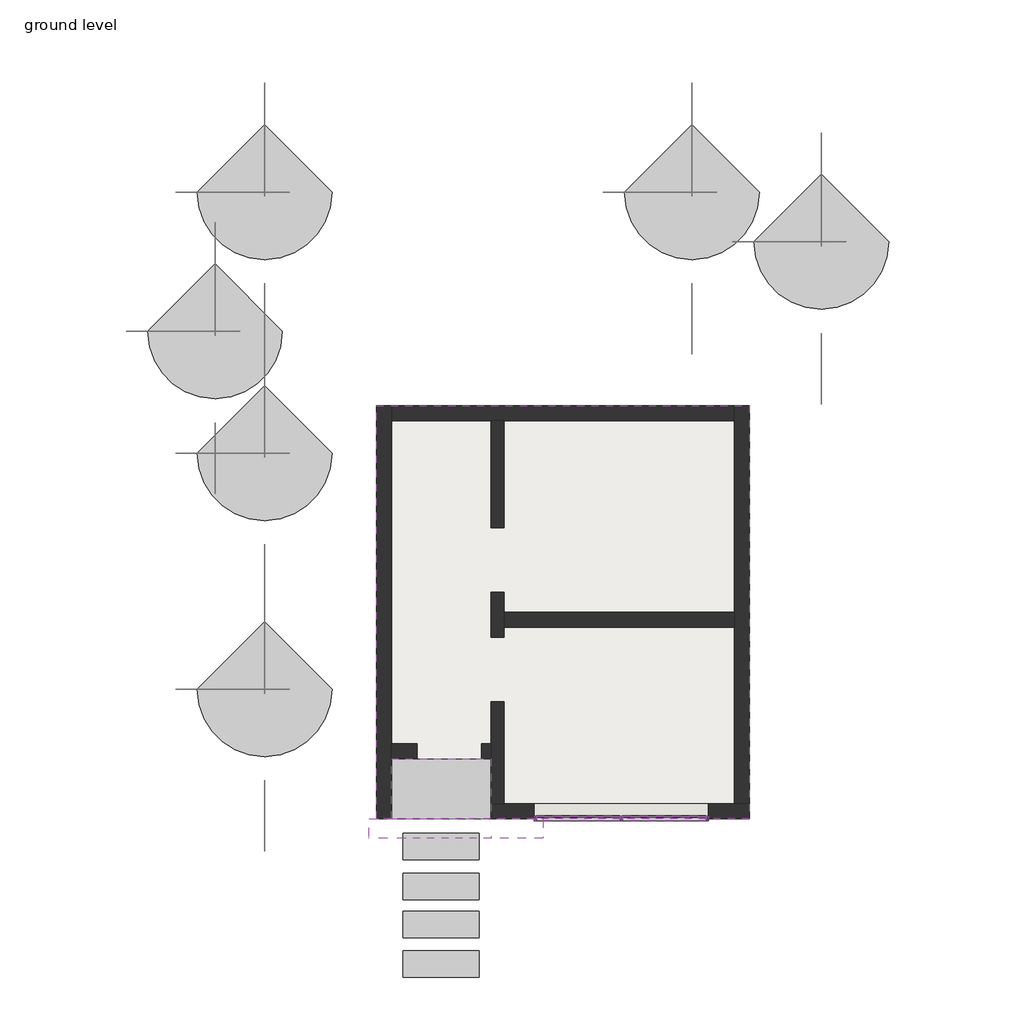
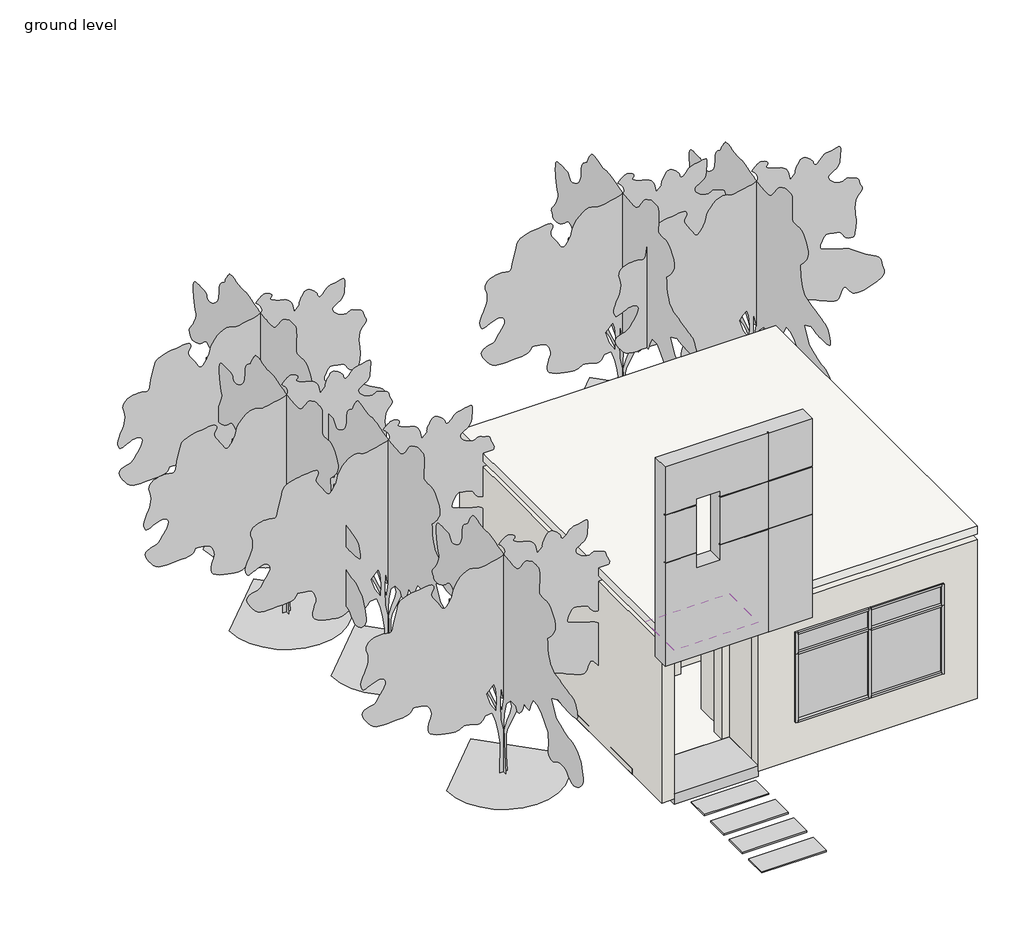
# One storey, incomplete: 12 members, 7 walls, 6 geographic elements, 4 plates, 3 proxies, 2 slabs, 1 covering.
"""IFC4 building model written with IfcOpenShell, lengths in millimetres."""

from ifc_helpers import new_model, si_unit, frame, origin, origin_with_axes, place, context, project, spatial, polyline, outline, extrude, faceted_brep, transform, mapped, element, save
from components import generic_models_2_generic_models_2_020848e7, generic_models_5_generic_models_5_6b2521d7, generic_models_6_generic_models_6_e57160bd, rpc_tree_deciduous_blue_berry_elder_15_a2d70376, member_9069d910, member_f8a7f713, member_03258ea9, member_54524429, member_711dd202, member_030f819f, system_panel_glazed_4e3b5d9d, system_panel_glazed_6984195a

model = new_model("IFC4")

# Units and contexts
model_context = context("Model", 3, world=origin())
ifc_project = project(units=[si_unit("LENGTHUNIT", "METRE", prefix="MILLI")], contexts=[model_context])

# Site, building, storey
site = spatial("IfcSite", under=ifc_project)
building = spatial("IfcBuilding", under=site)
storey = spatial("IfcBuildingStorey", under=building, Name="ground level", Elevation=0.0)

# Proxies
placement = place(None, origin())
generic_models_2_generic_models_2_shape = generic_models_2_generic_models_2_020848e7(model_context)
element("IfcBuildingElementProxy", 1, Name="Generic Models 2 : Generic Models 2", ObjectType="Generic Models 2 : Generic Models 2", at=placement, inside=storey, context=model_context, shape_type="MappedRepresentation", body=[
    mapped(generic_models_2_generic_models_2_shape, transform((0.0, 0.0, 0.0), x_axis=(1.0, 0.0, 0.0), y_axis=(0.0, 1.0, 0.0), z_axis=(0.0, 0.0, 1.0))),
])
generic_models_5_generic_models_5_shape = generic_models_5_generic_models_5_6b2521d7(model_context)
element("IfcBuildingElementProxy", 2, Name="Generic Models 5 : Generic Models 5", ObjectType="Generic Models 5 : Generic Models 5", at=placement, inside=storey, context=model_context, shape_type="MappedRepresentation", body=[
    mapped(generic_models_5_generic_models_5_shape, transform((0.0, 0.0, 0.0), x_axis=(1.0, 0.0, 0.0), y_axis=(0.0, 1.0, 0.0), z_axis=(0.0, 0.0, 1.0))),
])
generic_models_6_generic_models_6_shape = generic_models_6_generic_models_6_e57160bd(model_context)
element("IfcBuildingElementProxy", 3, Name="Generic Models 6 : Generic Models 6", ObjectType="Generic Models 6 : Generic Models 6", at=placement, inside=storey, context=model_context, shape_type="MappedRepresentation", body=[
    mapped(generic_models_6_generic_models_6_shape, transform((0.0, 0.0, 0.0), x_axis=(1.0, 0.0, 0.0), y_axis=(0.0, 1.0, 0.0), z_axis=(0.0, 0.0, 1.0))),
])

# Covering
element("IfcCovering", 4, ObjectType="2' x 4' ACT System", at=placement, inside=storey, context=model_context, shape_type="SweptSolid", body=[
    extrude(outline(polyline([(-9858.9678816, 2250.9030358), (-8334.9678816, 2250.9030358), (-8334.9678816, 1336.5030358), (-9858.9678816, 1336.5030358), (-9858.9678816, 2250.9030358)])), frame((0.0, 0.0, 2743.2), z_axis=(0.0, 0.0, 1.0), x_axis=(1.0, 0.0, 0.0)), (0.0, 0.0, 1.0), 57.15),
])

# Geographic elements
rpc_tree_deciduous_blue_berry_elder_15_shape = rpc_tree_deciduous_blue_berry_elder_15_a2d70376(model_context)
element("IfcGeographicElement", 5, ObjectType="RPC Tree - Deciduous : Blue Berry Elder - 15'", at=placement, inside=storey, context=model_context, shape_type="MappedRepresentation", body=[
    mapped(rpc_tree_deciduous_blue_berry_elder_15_shape, transform((-3267.6678816, 10175.7030358, -101.6), x_axis=(1.0, 0.0, 0.0), y_axis=(0.0, 1.0, 0.0), z_axis=(0.0, 0.0, 1.0))),
])
element("IfcGeographicElement", 6, ObjectType="RPC Tree - Deciduous : Blue Berry Elder - 15'", at=placement, inside=storey, context=model_context, shape_type="MappedRepresentation", body=[
    mapped(rpc_tree_deciduous_blue_berry_elder_15_shape, transform((-5248.8678816, 10937.7030358, -101.6), x_axis=(1.0, 0.0, 0.0), y_axis=(0.0, 1.0, 0.0), z_axis=(0.0, 0.0, 1.0))),
])
element("IfcGeographicElement", 7, ObjectType="RPC Tree - Deciduous : Blue Berry Elder - 15'", at=placement, inside=storey, context=model_context, shape_type="MappedRepresentation", body=[
    mapped(rpc_tree_deciduous_blue_berry_elder_15_shape, transform((-11802.0678816, 10937.7030358, -101.6), x_axis=(1.0, 0.0, 0.0), y_axis=(0.0, 1.0, 0.0), z_axis=(0.0, 0.0, 1.0))),
])
element("IfcGeographicElement", 8, ObjectType="RPC Tree - Deciduous : Blue Berry Elder - 15'", at=placement, inside=storey, context=model_context, shape_type="MappedRepresentation", body=[
    mapped(rpc_tree_deciduous_blue_berry_elder_15_shape, transform((-12564.0678816, 8804.1030358, -101.6), x_axis=(1.0, 0.0, 0.0), y_axis=(0.0, 1.0, 0.0), z_axis=(0.0, 0.0, 1.0))),
])
element("IfcGeographicElement", 9, ObjectType="RPC Tree - Deciduous : Blue Berry Elder - 15'", at=placement, inside=storey, context=model_context, shape_type="MappedRepresentation", body=[
    mapped(rpc_tree_deciduous_blue_berry_elder_15_shape, transform((-11802.0678816, 6937.2030358, -101.6), x_axis=(1.0, 0.0, 0.0), y_axis=(0.0, 1.0, 0.0), z_axis=(0.0, 0.0, 1.0))),
])
element("IfcGeographicElement", 10, ObjectType="RPC Tree - Deciduous : Blue Berry Elder - 15'", at=placement, inside=storey, context=model_context, shape_type="MappedRepresentation", body=[
    mapped(rpc_tree_deciduous_blue_berry_elder_15_shape, transform((-11802.0678816, 3317.7030358, -101.6), x_axis=(1.0, 0.0, 0.0), y_axis=(0.0, 1.0, 0.0), z_axis=(0.0, 0.0, 1.0))),
])

# Members
member_shape = member_9069d910(model_context)
element("IfcMember", 11, ObjectType="Rectangular Mullion : 1.5\" x 2.5\" rectangular", at=placement, inside=storey, context=model_context, shape_type="MappedRepresentation", body=[
    mapped(member_shape, transform((-5032.9678816, 1336.5030358, 2331.2360761), x_axis=(0.0, 0.0, 1.0), y_axis=(0.0, -1.0, 0.0), z_axis=(1.0, 0.0, 0.0))),
])
element("IfcMember", 12, ObjectType="Rectangular Mullion : 1.5\" x 2.5\" rectangular", at=placement, inside=storey, context=model_context, shape_type="MappedRepresentation", body=[
    mapped(member_shape, transform((-6353.7678816, 1336.5030358, 2331.2360761), x_axis=(0.0, 0.0, 1.0), y_axis=(0.0, -1.0, 0.0), z_axis=(1.0, 0.0, 0.0))),
])
element("IfcMember", 13, ObjectType="Rectangular Mullion : 1.5\" x 2.5\" rectangular", at=placement, inside=storey, context=model_context, shape_type="MappedRepresentation", body=[
    mapped(member_shape, transform((-7636.4678816, 1336.5030358, 609.6), x_axis=(0.0, 0.0, -1.0), y_axis=(0.0, -1.0, 0.0), z_axis=(-1.0, 0.0, 0.0))),
])
element("IfcMember", 14, ObjectType="Rectangular Mullion : 1.5\" x 2.5\" rectangular", at=placement, inside=storey, context=model_context, shape_type="MappedRepresentation", body=[
    mapped(member_shape, transform((-6315.6678816, 1336.5030358, 609.6), x_axis=(0.0, 0.0, -1.0), y_axis=(0.0, -1.0, 0.0), z_axis=(-1.0, 0.0, 0.0))),
])
member_2_shape = member_f8a7f713(model_context)
element("IfcMember", 15, ObjectType="Rectangular Mullion : 1.5\" x 2.5\" rectangular", at=placement, inside=storey, context=model_context, shape_type="MappedRepresentation", body=[
    mapped(member_2_shape, transform((-6334.7178816, 1336.5030358, 609.6), x_axis=(1.0, 0.0, 0.0), y_axis=(0.0, -1.0, 0.0), z_axis=(0.0, 0.0, -1.0))),
])
member_3_shape = member_03258ea9(model_context)
element("IfcMember", 16, ObjectType="Rectangular Mullion : 1.5\" x 2.5\" rectangular", at=placement, inside=storey, context=model_context, shape_type="MappedRepresentation", body=[
    mapped(member_3_shape, transform((-6353.7678816, 1336.5030358, 1924.8360761), x_axis=(0.0, 0.0, 1.0), y_axis=(0.0, -1.0, 0.0), z_axis=(1.0, 0.0, 0.0))),
])
element("IfcMember", 17, ObjectType="Rectangular Mullion : 1.5\" x 2.5\" rectangular", at=placement, inside=storey, context=model_context, shape_type="MappedRepresentation", body=[
    mapped(member_3_shape, transform((-5032.9678816, 1336.5030358, 1924.8360761), x_axis=(0.0, 0.0, 1.0), y_axis=(0.0, -1.0, 0.0), z_axis=(1.0, 0.0, 0.0))),
])
member_4_shape = member_54524429(model_context)
element("IfcMember", 18, ObjectType="Rectangular Mullion : 1.5\" x 2.5\" rectangular", at=placement, inside=storey, context=model_context, shape_type="MappedRepresentation", body=[
    mapped(member_4_shape, transform((-6334.7178816, 1336.5030358, 1924.8360761), x_axis=(1.0, 0.0, 0.0), y_axis=(0.0, -1.0, 0.0), z_axis=(0.0, 0.0, -1.0))),
])
member_5_shape = member_711dd202(model_context)
element("IfcMember", 19, ObjectType="Rectangular Mullion : 1.5\" x 2.5\" rectangular", at=placement, inside=storey, context=model_context, shape_type="MappedRepresentation", body=[
    mapped(member_5_shape, transform((-7674.5678816, 1336.5030358, 2331.2360761), x_axis=(-1.0, 0.0, 0.0), y_axis=(0.0, -1.0, 0.0), z_axis=(0.0, 0.0, 1.0))),
])
member_6_shape = member_030f819f(model_context)
element("IfcMember", 20, ObjectType="Rectangular Mullion : 1.5\" x 2.5\" rectangular", at=placement, inside=storey, context=model_context, shape_type="MappedRepresentation", body=[
    mapped(member_6_shape, transform((-4994.8678816, 1336.5030358, 609.6), x_axis=(1.0, 0.0, 0.0), y_axis=(0.0, -1.0, 0.0), z_axis=(0.0, 0.0, -1.0))),
])
element("IfcMember", 21, ObjectType="Rectangular Mullion : 1.5\" x 2.5\" rectangular", at=placement, inside=storey, context=model_context, shape_type="MappedRepresentation", body=[
    mapped(member_5_shape, transform((-4994.8678816, 1336.5030358, 1924.8360761), x_axis=(1.0, 0.0, 0.0), y_axis=(0.0, -1.0, 0.0), z_axis=(0.0, 0.0, -1.0))),
])
element("IfcMember", 22, ObjectType="Rectangular Mullion : 1.5\" x 2.5\" rectangular", at=placement, inside=storey, context=model_context, shape_type="MappedRepresentation", body=[
    mapped(member_6_shape, transform((-7674.5678816, 1336.5030358, 1924.8360761), x_axis=(-1.0, 0.0, 0.0), y_axis=(0.0, -1.0, 0.0), z_axis=(0.0, 0.0, 1.0))),
])

# Plates
system_panel_glazed_shape = system_panel_glazed_4e3b5d9d(model_context)
element("IfcPlate", 23, ObjectType="System Panel : Glazed", at=placement, inside=storey, context=model_context, shape_type="MappedRepresentation", body=[
    mapped(system_panel_glazed_shape, transform((-6995.1178816, 1336.5030358, 647.7), x_axis=(1.0, 0.0, 0.0), y_axis=(0.0, 1.0, 0.0), z_axis=(0.0, 0.0, 1.0))),
])
element("IfcPlate", 24, ObjectType="System Panel : Glazed", at=placement, inside=storey, context=model_context, shape_type="MappedRepresentation", body=[
    mapped(system_panel_glazed_shape, transform((-5674.3178816, 1336.5030358, 647.7), x_axis=(1.0, 0.0, 0.0), y_axis=(0.0, 1.0, 0.0), z_axis=(0.0, 0.0, 1.0))),
])
system_panel_glazed_2_shape = system_panel_glazed_6984195a(model_context)
element("IfcPlate", 25, ObjectType="System Panel : Glazed", at=placement, inside=storey, context=model_context, shape_type="MappedRepresentation", body=[
    mapped(system_panel_glazed_2_shape, transform((-6995.1178816, 1336.5030358, 1943.8860761), x_axis=(1.0, 0.0, 0.0), y_axis=(0.0, 1.0, 0.0), z_axis=(0.0, 0.0, 1.0))),
])
element("IfcPlate", 26, ObjectType="System Panel : Glazed", at=placement, inside=storey, context=model_context, shape_type="MappedRepresentation", body=[
    mapped(system_panel_glazed_2_shape, transform((-5674.3178816, 1336.5030358, 1943.8860761), x_axis=(1.0, 0.0, 0.0), y_axis=(0.0, 1.0, 0.0), z_axis=(0.0, 0.0, 1.0))),
])

# Slabs
element("IfcSlab", 27, ObjectType="Generic - 4\"", at=placement, inside=storey, context=model_context, shape_type="SweptSolid", body=[
    extrude(outline(polyline([(-4372.5678816, 7661.1030358), (-4372.5678816, 1565.1030358), (-8334.9678816, 1565.1030358), (-8334.9678816, 2250.9030358), (-10087.5678816, 2250.9030358), (-10087.5678816, 7661.1030358), (-4372.5678816, 7661.1030358)])), frame((0.0, 0.0, -101.6), z_axis=(0.0, 0.0, 1.0), x_axis=(1.0, 0.0, 0.0)), (0.0, 0.0, 1.0), 101.6),
])
element("IfcSlab", 28, ObjectType="Generic - 6\"", at=placement, inside=storey, context=model_context, shape_type="SweptSolid", body=[
    extrude(outline(polyline([(-4372.5678816, 7661.1030358), (-4372.5678816, 1336.5030358), (-10087.5678816, 1336.5030358), (-10087.5678816, 7661.1030358), (-4372.5678816, 7661.1030358)])), frame((0.0, 0.0, 3048.0), z_axis=(0.0, 0.0, 1.0), x_axis=(1.0, 0.0, 0.0)), (0.0, 0.0, 1.0), 152.4),
])

# Walls
element("IfcWall", 29, ObjectType="Generic - 4.5\"", at=placement, inside=storey, context=model_context, shape_type="Brep", body=[
    faceted_brep([(-8334.9678816, 1565.1030358, 3048.0), (-8334.9678816, 2250.9030358, 3048.0), (-8334.9678816, 2479.5030358, 3048.0), (-8334.9678816, 7432.5030358, 3048.0), (-8334.9678816, 7432.5030358, 0.0), (-8334.9678816, 5794.2030358, 0.0), (-8334.9678816, 5794.2030358, 2133.6), (-8334.9678816, 4803.6030358, 2133.6), (-8334.9678816, 4803.6030358, 0.0), (-8334.9678816, 4117.8030358, 0.0), (-8334.9678816, 4117.8030358, 2133.6), (-8334.9678816, 3127.2030358, 2133.6), (-8334.9678816, 3127.2030358, 0.0), (-8334.9678816, 2479.5030358, 0.0), (-8334.9678816, 2250.9030358, 0.0), (-8334.9678816, 1565.1030358, 0.0), (-8334.9678816, 1565.1030358, 2946.4), (-8131.7678816, 7432.5030358, 3048.0), (-8131.7678816, 4498.8030358, 3048.0), (-8131.7678816, 4270.2030358, 3048.0), (-8131.7678816, 1565.1030358, 3048.0), (-8131.7678816, 1565.1030358, 0.0), (-8131.7678816, 3127.2030358, 0.0), (-8131.7678816, 3127.2030358, 2133.6), (-8131.7678816, 4117.8030358, 2133.6), (-8131.7678816, 4117.8030358, 0.0), (-8131.7678816, 4270.2030358, 0.0), (-8131.7678816, 4498.8030358, 0.0), (-8131.7678816, 4803.6030358, 0.0), (-8131.7678816, 4803.6030358, 2133.6), (-8131.7678816, 5794.2030358, 2133.6), (-8131.7678816, 5794.2030358, 0.0), (-8131.7678816, 7432.5030358, 0.0)], [[[0, 1, 2, 3, 4, 5, 6, 7, 8, 9, 10, 11, 12, 13, 14, 15, 16]], [[17, 18, 19, 20, 21, 22, 23, 24, 25, 26, 27, 28, 29, 30, 31, 32]], [[4, 32, 31, 5]], [[8, 28, 27, 26, 25, 9]], [[21, 15, 14, 13, 12, 22]], [[3, 2, 1, 0, 20, 19, 18, 17]], [[4, 3, 17, 32]], [[8, 7, 29, 28]], [[7, 6, 30, 29]], [[6, 5, 31, 30]], [[24, 10, 9, 25]], [[10, 24, 23, 11]], [[11, 23, 22, 12]], [[0, 16, 15, 21, 20]]]),
])
element("IfcWall", 30, ObjectType="Generic - 9\"", at=placement, inside=storey, context=model_context, shape_type="Brep", body=[
    faceted_brep([(-10087.5678816, 7661.1030358, -101.6), (-10087.5678816, 1336.5030358, -101.6), (-10087.5678816, 1336.5030358, 2946.4), (-10087.5678816, 7661.1030358, 2946.4), (-9858.9678816, 7661.1030358, -101.6), (-9858.9678816, 7661.1030358, 0.0), (-9858.9678816, 7661.1030358, 2946.4), (-9858.9678816, 1336.5030358, 2946.4), (-9858.9678816, 1336.5030358, -101.6)], [[[0, 1, 2, 3]], [[4, 5, 6, 7, 8]], [[1, 0, 4, 8]], [[2, 1, 8, 7]], [[3, 2, 7, 6]], [[0, 3, 6, 5, 4]]]),
])
element("IfcWall", 31, ObjectType="Generic - 9\"", at=placement, inside=storey, context=model_context, shape_type="Brep", body=[
    faceted_brep([(-8334.9678816, 1336.5030358, -101.6), (-4372.5678816, 1336.5030358, -101.6), (-4372.5678816, 1336.5030358, 2946.4), (-8334.9678816, 1336.5030358, 2946.4), (-7674.5678816, 1336.5030358, 2331.2360761), (-4994.8678816, 1336.5030358, 2331.2360761), (-4994.8678816, 1336.5030358, 609.6), (-7674.5678816, 1336.5030358, 609.6), (-4372.5678816, 1565.1030358, -101.6), (-8334.9678816, 1565.1030358, -101.6), (-8334.9678816, 1565.1030358, 0.0), (-8334.9678816, 1565.1030358, 2946.4), (-4372.5678816, 1565.1030358, 2946.4), (-4372.5678816, 1565.1030358, 0.0), (-4994.8678816, 1565.1030358, 2331.2360761), (-7674.5678816, 1565.1030358, 2331.2360761), (-7674.5678816, 1565.1030358, 609.6), (-4994.8678816, 1565.1030358, 609.6)], [[[0, 1, 2, 3], [4, 5, 6, 7]], [[8, 9, 10, 11, 12, 13], [14, 15, 16, 17]], [[1, 0, 9, 8]], [[3, 2, 12, 11]], [[2, 1, 8, 13, 12]], [[4, 15, 14, 5]], [[6, 17, 16, 7]], [[15, 4, 7, 16]], [[5, 14, 17, 6]], [[0, 3, 11, 10, 9]]]),
])
element("IfcWall", 32, ObjectType="Generic - 9\"", at=placement, inside=storey, context=model_context, shape_type="Brep", body=[
    faceted_brep([(-4372.5678816, 1565.1030358, 0.0), (-4372.5678816, 7661.1030358, 0.0), (-4372.5678816, 7661.1030358, 3048.0), (-4372.5678816, 1565.1030358, 3048.0), (-4372.5678816, 1565.1030358, 2946.4), (-4601.1678816, 1565.1030358, 0.0), (-4601.1678816, 1565.1030358, 3048.0), (-4601.1678816, 4270.2030358, 3048.0), (-4601.1678816, 4498.8030358, 3048.0), (-4601.1678816, 7432.5030358, 3048.0), (-4601.1678816, 7661.1030358, 3048.0), (-4601.1678816, 7661.1030358, 0.0), (-4601.1678816, 7432.5030358, 0.0), (-4601.1678816, 4498.8030358, 0.0), (-4601.1678816, 4270.2030358, 0.0)], [[[0, 1, 2, 3, 4]], [[5, 6, 7, 8, 9, 10, 11, 12, 13, 14]], [[1, 0, 5, 14, 13, 12, 11]], [[3, 2, 10, 9, 8, 7, 6]], [[0, 4, 3, 6, 5]], [[2, 1, 11, 10]]]),
])
element("IfcWall", 33, ObjectType="Generic - 9\"", at=placement, inside=storey, context=model_context, shape_type="Brep", body=[
    faceted_brep([(-4601.1678816, 7661.1030358, 0.0), (-9858.9678816, 7661.1030358, 0.0), (-9858.9678816, 7661.1030358, 2946.4), (-9858.9678816, 7661.1030358, 3048.0), (-4601.1678816, 7661.1030358, 3048.0), (-4601.1678816, 7432.5030358, 0.0), (-4601.1678816, 7432.5030358, 3048.0), (-8131.7678816, 7432.5030358, 3048.0), (-8334.9678816, 7432.5030358, 3048.0), (-9858.9678816, 7432.5030358, 3048.0), (-9858.9678816, 7432.5030358, 0.0), (-8334.9678816, 7432.5030358, 0.0), (-8131.7678816, 7432.5030358, 0.0)], [[[0, 1, 2, 3, 4]], [[5, 6, 7, 8, 9, 10, 11, 12]], [[1, 0, 5, 12, 11, 10]], [[4, 3, 9, 8, 7, 6]], [[3, 2, 1, 10, 9]], [[0, 4, 6, 5]]]),
])
element("IfcWall", 34, ObjectType="Generic - 9\"", at=placement, inside=storey, context=model_context, shape_type="SweptSolid", body=[
    extrude(outline(polyline([(3048.0, -8334.9678816), (3048.0, -9858.9678816), (0.0, -9858.9678816), (0.0, -9465.2678816), (2133.6, -9465.2678816), (2133.6, -8474.6678816), (0.0, -8474.6678816), (0.0, -8334.9678816), (3048.0, -8334.9678816)])), frame((0.0, 2250.9030358, 0.0), z_axis=(0.0, 1.0, 0.0), x_axis=(0.0, 0.0, 1.0)), (0.0, 0.0, 1.0), 228.6),
])
element("IfcWall", 35, ObjectType="Generic - 9\"", at=placement, inside=storey, context=model_context, shape_type="SweptSolid", body=[
    extrude(outline(polyline([(-8131.7678816, 4498.8030358), (-4601.1678816, 4498.8030358), (-4601.1678816, 4270.2030358), (-8131.7678816, 4270.2030358), (-8131.7678816, 4498.8030358)])), origin_with_axes(), (0.0, 0.0, 1.0), 3048.0),
])

save(model, "model.ifc")

# Revit data of these elements
# Type "2' x 4' ACT System"
#   Assembly Code = "C3030210"
#   built-in parameter 1002203 = 1 (stored number, unit not read)
#   built-in parameter 1002202 = 1 (stored number, unit not read)
#   Layers, outside or top first: 0' - 1 5/8" "Default" (function 1); 0' - 0 5/8" "Acoustic Ceiling Tile 24 x 48" (function 5)
# Type "RPC Tree - Deciduous : Blue Berry Elder - 15'"
#   built-in parameter 1005198 = "{2, 15},{39, RPC-16-FWVX-4SXX-5R2N-A000-ST1L-LVER-AU},{1, 0},{1, 0},{2, 35},{1, 8},{5, Color},{1, 0},{1, 0},{3, 0.8},{3, 0.8},{3, 0.8},{1, 8},{7, BBoxMin},{1, 0},{1, 0},{1, 0},{1, 0},{1, 0},{1, 8},{7, BBoxMax},{1, 0},{1, 0},{1, 0},{1, 0},{1, 0},{2, 11},{9, RPCTypeId},{1, 0},{1, 0},{39, RPC-16-FWVX-4SXX-5R2N-A000-ST1L-LVER-AU},{1, 6},{14, RPCPlantHeight},{1, 0},{1, 0},{2, 15},{2, 11},{7, keyword},{1, 0},{1, 0},{285, :Geometry:RPC:Blue-Berry Elder:Sambucus cerulea:Tall:irregularly shaped shrubs or very small trees:up to 10 m high and 20 cm in diameter.  The larger of the Canadian elders; occurs in southern British Columbia in forest clearings:usually on dry open sites with gravelly or stony soils.},{2, 11},{8, category},{1, 0},{1, 0},{16, :Trees [General]},{2, 11},{12, LocalizedUID},{1, 0},{1, 0},{16, Blue-Berry Elder},{2, 14},{6, Height},{1, 0},{1, 0},{2, 15},{1, 2},{16, Cast Reflections},{1, 0},{1, 0},{1, 0},{1, 2},{12, Cast Shadows},{1, 0},{1, 0},{1, 1},{1, 2},{9, Lock View},{1, 0},{1, 0},{1, 0},{1, 4},{5, ViewC},{1, 0},{1, 0},{1, 0},{2, 11},{20, AdvancedUIDefinition},{1, 0},{1, 0},{0, },{2, 11},{10, AssetLibID},{1, 0},{1, 0},{36, 4D3F6E72-3F99-4203-98E9-AF80B3C7A7A4},{2, 11},{10, BaseSchema},{1, 0},{1, 0},{9, RPCSchema},{2, 11},{12, ExchangeGUID},{1, 0},{1, 0},{0, },{1, 2},{6, Hidden},{1, 0},{1, 0},{1, 0},{1, 4},{11, RPCCategory},{1, 0},{1, 0},{1, 0},{2, 11},{8, RPCImage},{1, 0},{1, 0},{0, },{1, 4},{13, SchemaVersion},{1, 0},{1, 0},{1, 4},{2, 11},{12, UIDefinition},{1, 0},{1, 0},{0, },{2, 11},{6, UIName},{1, 0},{1, 0},{39, RPC-16-FWVX-4SXX-5R2N-A000-ST1L-LVER-AU},{2, 11},{11, VersionGUID},{1, 0},{1, 0},{9, RPCSchema},{2, 11},{9, assettype},{1, 0},{1, 0},{11, RPCGeometry},{2, 11},{11, description},{1, 0},{1, 0},{0, },{2, 11},{9, localname},{1, 0},{1, 0},{3, RPC},{2, 11},{9, localtype},{1, 0},{1, 0},{3, RPC},{1, 4},{8, revision},{1, 0},{1, 0},{1, 1},{2, 11},{9, thumbnail},{1, 0},{1, 0},{0, },{1, 4},{7, version},{1, 0},{1, 0},{1, 1},{1, 2},{20, RPC_Cast Reflections},{1, 0},{1, 0},{1, 1},{1, 2},{16, RPC_Cast Shadows},{1, 0},{1, 0},{1, 1},{1, 2},{13, RPC_Lock View},{1, 0},{1, 0},{1, 0},{1, 4},{9, RPC_ViewC},{1, 0},{1, 0},{1, 0},{21, assetlibrary_base.fbx},{1, 5},"
#   built-in parameter 1005195 = "RPC-16-FWVX-4SXX-5R2N-A000-ST1L-LVER-AU"
#   Type Comments = "Blue Berry Elder"
#   Assembly Code = "G2050500"
#   Height = 15' - 0"
#   Default Elevation = 0
# Type "Rectangular Mullion : 1.5\" x 2.5\" rectangular"
#   built-in parameter 1007304 = 0.208333 (stored number, unit not read)
#   built-in parameter 1007301 = 0.0625 (stored number, unit not read)
#   built-in parameter 1007300 = 0.0625 (stored number, unit not read)
# Type "System Panel : Glazed"
#   Construction Type Id = "GSP4R"
#   Analytic Construction = "1/8 in Pilkington single glazing"
#   Visual Light Transmittance = 0.9
#   Solar Heat Gain Coefficient = 0.86
#   Heat Transfer Coefficient (U) = 1.18115 BTU/(h·ft²·°F)
#   Define Thermal Properties by = 1
# Type "Generic - 4\""
#   Assembly Code = "B1010"
#   Function = 0
#   Layers, outside or top first: 0' - 4" no material (function 1)
# Type "Generic - 6\""
#   Assembly Code = "B1010"
#   Function = 0
#   Layers, outside or top first: 0' - 6" no material (function 1)
# Type "Generic - 4.5\""
#   Assembly Code = "B2010"
#   Layers, outside or top first: 0' - 8" no material (function 1)
# Type "Generic - 9\""
#   Assembly Code = "B2010"
#   Layers, outside or top first: 0' - 9" no material (function 1)
# Element 1 (IfcBuildingElementProxy, "Generic Models 2 : Generic Models 2")
#   Phase Created = New Construction
#   Materials on its faces: "wall paint"
# Element 2 (IfcBuildingElementProxy, "Generic Models 5 : Generic Models 5")
#   Phase Created = New Construction
#   Materials on its faces: "Concrete, Cast-in-Place gray"
# Element 3 (IfcBuildingElementProxy, "Generic Models 6 : Generic Models 6")
#   Phase Created = New Construction
#   Materials on its faces: "Concrete, Cast-in-Place gray"
# Element 4 (IfcCovering, "2' x 4' ACT System")
#   Height Offset From Level = 9' - 0"
#   Phase Created = New Construction
#   Materials on its faces: "Acoustic Ceiling Tile 24 x 48", "Default"
# Elements 5, 6, 7, 8, 9, 10 (IfcGeographicElement, "RPC Tree - Deciduous : Blue Berry Elder - 15'")
#   Phase Created = New Construction
# Elements 11, 12, 13, 14, 15, 16, 17, 18, 19, 20, 21, 22 (IfcMember, "Rectangular Mullion : 1.5\" x 2.5\" rectangular")
#   Phase Created = New Construction
#   Materials on its faces: "Damp-proofing"
# Elements 23, 24, 25, 26 (IfcPlate, "System Panel : Glazed")
#   Phase Created = New Construction
#   Materials on its faces: "Glass"
# Element 27 (IfcSlab, "Generic - 4\"")
#   Height Offset From Level = 0' - 0"
#   Phase Created = New Construction
#   Materials on its faces: "Default Floor"
# Element 28 (IfcSlab, "Generic - 6\"")
#   Height Offset From Level = 10' - 6"
#   Phase Created = New Construction
#   Materials on its faces: "Default Floor", "wall paint"
# Element 29 (IfcWall, "Generic - 4.5\"")
#   Top Offset = 0' - 0"
#   Base Offset = 0' - 0"
#   Unconnected Height = 10' - 0"
#   wall height = 10' - 0"
#   Phase Created = New Construction
#   Base Constraint = ground level
#   Materials on its faces: "Default Wall", "wall paint"
# Element 30 (IfcWall, "Generic - 9\"")
#   built-in parameter 1001111 = -0' - 4"
#   Top Offset = 0' - 0"
#   Base Offset = -0' - 4"
#   Unconnected Height = 10' - 0"
#   wall height = 10' - 0"
#   Phase Created = New Construction
#   Base Constraint = ground level
#   Materials on its faces: "wall paint", "Default Wall"
# Element 31 (IfcWall, "Generic - 9\"")
#   built-in parameter 1001111 = -0' - 4"
#   Top Offset = 0' - 0"
#   Base Offset = -0' - 4"
#   Unconnected Height = 10' - 0"
#   wall height = 10' - 0"
#   Phase Created = New Construction
#   Base Constraint = ground level
#   Materials on its faces: "Default Wall", "wall paint"
# Elements 32, 34 (IfcWall, "Generic - 9\"")
#   Top Offset = 0' - 0"
#   Base Offset = 0' - 0"
#   Unconnected Height = 10' - 0"
#   wall height = 10' - 0"
#   Phase Created = New Construction
#   Base Constraint = ground level
#   Materials on its faces: "Default Wall", "wall paint"
# Elements 33, 35 (IfcWall, "Generic - 9\"")
#   Top Offset = 0' - 0"
#   Base Offset = 0' - 0"
#   Unconnected Height = 10' - 0"
#   wall height = 10' - 0"
#   Phase Created = New Construction
#   Base Constraint = ground level
#   Materials on its faces: "Default Wall"
# Materials
#   "Default": colour RGB 127 127 127, transparency 0, Cost = 0
#   "Acoustic Ceiling Tile 24 x 48": class "Generic", colour RGB 229 229 229, transparency 0, Description = "Acoustic Ceiling Tile 24 x 48", Cost = 0
#   "wall paint": class "Generic", colour RGB 120 120 120, transparency 0, Cost = 0
#   "Concrete, Cast-in-Place gray": class "Concrete", colour RGB 192 192 192, transparency 0, Description = "Cast-in-place concrete", Cost = 0
#   "Damp-proofing": class "Generic", colour RGB 127 127 127, transparency 0, Description = "Damp-proofing", Cost = 0
#   "Glass": class "Glass", colour RGB 0 128 192, transparency 0.75, Description = "Soda Lime Glass", Cost = 0
#   "Default Floor": colour RGB 128 128 128, transparency 0, Cost = 0
#   "Default Wall": colour RGB 128 128 128, transparency 0, Cost = 0
